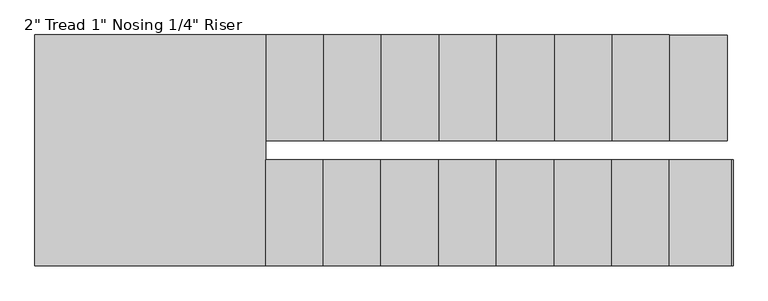
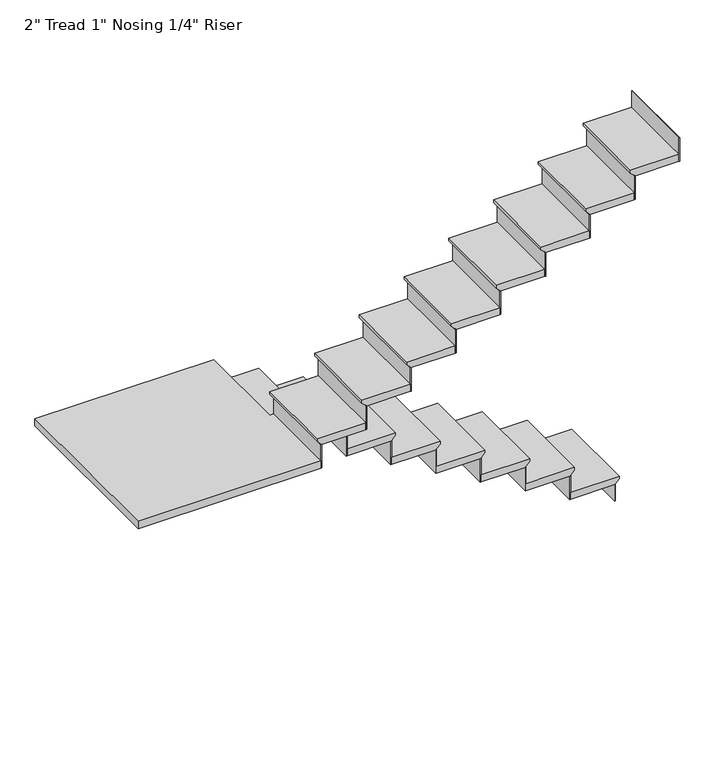
"""IFC4 building model written with IfcOpenShell, lengths in millimetres: stair flight geometry."""

from ifc_helpers import new_model, si_unit, origin, place, context, project, spatial, faceted_brep, source, transform, mapped, element, save


def stair_flight_719863f8(model_context):
    return source(origin(), model_context, "Body", "Brep", [
        faceted_brep([(-1805.9198569, -5306.3933037, 6551.0833333), (-1805.9198569, -5306.3933037, 6570.1333333), (-1805.9198569, -5865.1933037, 6570.1333333), (-1805.9198569, -5865.1933037, 6551.0833333), (-1831.3198569, -5306.3933037, 6525.6833333), (-1831.3198569, -5865.1933037, 6525.6833333), (-2136.1198569, -5306.3933037, 6570.1333333), (-2136.1198569, -5865.1933037, 6570.1333333), (-1831.3198569, -5865.1933037, 6519.3333333), (-2136.1198569, -5865.1933037, 6519.3333333), (-2136.1198569, -5306.3933037, 6519.3333333), (-1831.3198569, -5306.3933037, 6519.3333333)], [[[0, 1, 2, 3]], [[4, 0, 3, 5]], [[2, 1, 6, 7]], [[8, 9, 10, 11]], [[2, 7, 9, 8, 5, 3]], [[8, 11, 4, 5]], [[6, 1, 0, 4, 11, 10]], [[7, 6, 10, 9]]]),
        faceted_brep([(-1831.3198569, -5306.3933037, 6519.3333333), (-1831.3198569, -5306.3933037, 6400.8), (-1837.6698569, -5306.3933037, 6400.8), (-1837.6698569, -5306.3933037, 6519.3333333), (-1831.3198569, -5865.1933037, 6519.3333333), (-1837.6698569, -5865.1933037, 6519.3333333), (-1837.6698569, -5865.1933037, 6400.8), (-1831.3198569, -5865.1933037, 6400.8)], [[[0, 1, 2, 3]], [[4, 5, 6, 7]], [[1, 0, 4, 7]], [[2, 1, 7, 6]], [[3, 2, 6, 5]], [[0, 3, 5, 4]]]),
        faceted_brep([(-2136.1198569, -5306.3933037, 6688.6666667), (-2136.1198569, -5306.3933037, 6519.3333333), (-2142.4698569, -5306.3933037, 6519.3333333), (-2142.4698569, -5306.3933037, 6688.6666667), (-2136.1198569, -5865.1933037, 6688.6666667), (-2142.4698569, -5865.1933037, 6688.6666667), (-2142.4698569, -5865.1933037, 6519.3333333), (-2136.1198569, -5865.1933037, 6519.3333333)], [[[0, 1, 2, 3]], [[4, 5, 6, 7]], [[1, 0, 4, 7]], [[2, 1, 7, 6]], [[3, 2, 6, 5]], [[0, 3, 5, 4]]]),
        faceted_brep([(-2110.7198569, -5865.1933037, 6739.4666667), (-2110.7198569, -5306.3933037, 6739.4666667), (-2440.9198569, -5306.3933037, 6739.4666667), (-2440.9198569, -5865.1933037, 6739.4666667), (-2136.1198569, -5865.1933037, 6688.6666667), (-2440.9198569, -5865.1933037, 6688.6666667), (-2440.9198569, -5306.3933037, 6688.6666667), (-2136.1198569, -5306.3933037, 6688.6666667), (-2136.1198569, -5865.1933037, 6695.0166667), (-2110.7198569, -5865.1933037, 6720.4166667), (-2136.1198569, -5306.3933037, 6695.0166667), (-2110.7198569, -5306.3933037, 6720.4166667)], [[[0, 1, 2, 3]], [[4, 5, 6, 7]], [[0, 3, 5, 4, 8, 9]], [[4, 7, 10, 8]], [[2, 1, 11, 10, 7, 6]], [[3, 2, 6, 5]], [[11, 1, 0, 9]], [[10, 11, 9, 8]]]),
        faceted_brep([(-2440.9198569, -5306.3933037, 6858.0), (-2440.9198569, -5306.3933037, 6688.6666667), (-2447.2698569, -5306.3933037, 6688.6666667), (-2447.2698569, -5306.3933037, 6858.0), (-2440.9198569, -5865.1933037, 6858.0), (-2447.2698569, -5865.1933037, 6858.0), (-2447.2698569, -5865.1933037, 6688.6666667), (-2440.9198569, -5865.1933037, 6688.6666667)], [[[0, 1, 2, 3]], [[4, 5, 6, 7]], [[1, 0, 4, 7]], [[2, 1, 7, 6]], [[3, 2, 6, 5]], [[0, 3, 5, 4]]]),
        faceted_brep([(-2415.5198569, -5865.1933037, 6908.8), (-2415.5198569, -5306.3933037, 6908.8), (-2745.7198569, -5306.3933037, 6908.8), (-2745.7198569, -5865.1933037, 6908.8), (-2440.9198569, -5865.1933037, 6858.0), (-2745.7198569, -5865.1933037, 6858.0), (-2745.7198569, -5306.3933037, 6858.0), (-2440.9198569, -5306.3933037, 6858.0), (-2440.9198569, -5865.1933037, 6864.35), (-2415.5198569, -5865.1933037, 6889.75), (-2440.9198569, -5306.3933037, 6864.35), (-2415.5198569, -5306.3933037, 6889.75)], [[[0, 1, 2, 3]], [[4, 5, 6, 7]], [[0, 3, 5, 4, 8, 9]], [[4, 7, 10, 8]], [[2, 1, 11, 10, 7, 6]], [[3, 2, 6, 5]], [[11, 1, 0, 9]], [[10, 11, 9, 8]]]),
        faceted_brep([(-2745.7198569, -5306.3933037, 7027.3333333), (-2745.7198569, -5306.3933037, 6858.0), (-2752.0698569, -5306.3933037, 6858.0), (-2752.0698569, -5306.3933037, 7027.3333333), (-2745.7198569, -5865.1933037, 7027.3333333), (-2752.0698569, -5865.1933037, 7027.3333333), (-2752.0698569, -5865.1933037, 6858.0), (-2745.7198569, -5865.1933037, 6858.0)], [[[0, 1, 2, 3]], [[4, 5, 6, 7]], [[1, 0, 4, 7]], [[2, 1, 7, 6]], [[3, 2, 6, 5]], [[0, 3, 5, 4]]]),
        faceted_brep([(-2720.3198569, -5865.1933037, 7078.1333333), (-2720.3198569, -5306.3933037, 7078.1333333), (-3050.5198569, -5306.3933037, 7078.1333333), (-3050.5198569, -5865.1933037, 7078.1333333), (-2745.7198569, -5865.1933037, 7027.3333333), (-3050.5198569, -5865.1933037, 7027.3333333), (-3050.5198569, -5306.3933037, 7027.3333333), (-2745.7198569, -5306.3933037, 7027.3333333), (-2745.7198569, -5865.1933037, 7033.6833333), (-2720.3198569, -5865.1933037, 7059.0833333), (-2745.7198569, -5306.3933037, 7033.6833333), (-2720.3198569, -5306.3933037, 7059.0833333)], [[[0, 1, 2, 3]], [[4, 5, 6, 7]], [[0, 3, 5, 4, 8, 9]], [[4, 7, 10, 8]], [[2, 1, 11, 10, 7, 6]], [[3, 2, 6, 5]], [[11, 1, 0, 9]], [[10, 11, 9, 8]]]),
        faceted_brep([(-3050.5198569, -5306.3933037, 7196.6666667), (-3050.5198569, -5306.3933037, 7027.3333333), (-3056.8698569, -5306.3933037, 7027.3333333), (-3056.8698569, -5306.3933037, 7196.6666667), (-3050.5198569, -5865.1933037, 7196.6666667), (-3056.8698569, -5865.1933037, 7196.6666667), (-3056.8698569, -5865.1933037, 7027.3333333), (-3050.5198569, -5865.1933037, 7027.3333333)], [[[0, 1, 2, 3]], [[4, 5, 6, 7]], [[1, 0, 4, 7]], [[2, 1, 7, 6]], [[3, 2, 6, 5]], [[0, 3, 5, 4]]]),
        faceted_brep([(-3025.1198569, -5865.1933037, 7247.4666667), (-3025.1198569, -5306.3933037, 7247.4666667), (-3355.3198569, -5306.3933037, 7247.4666667), (-3355.3198569, -5865.1933037, 7247.4666667), (-3050.5198569, -5865.1933037, 7196.6666667), (-3355.3198569, -5865.1933037, 7196.6666667), (-3355.3198569, -5306.3933037, 7196.6666667), (-3050.5198569, -5306.3933037, 7196.6666667), (-3050.5198569, -5865.1933037, 7203.0166667), (-3025.1198569, -5865.1933037, 7228.4166667), (-3050.5198569, -5306.3933037, 7203.0166667), (-3025.1198569, -5306.3933037, 7228.4166667)], [[[0, 1, 2, 3]], [[4, 5, 6, 7]], [[0, 3, 5, 4, 8, 9]], [[4, 7, 10, 8]], [[2, 1, 11, 10, 7, 6]], [[3, 2, 6, 5]], [[11, 1, 0, 9]], [[10, 11, 9, 8]]]),
        faceted_brep([(-3355.3198569, -5306.3933037, 7366.0), (-3355.3198569, -5306.3933037, 7196.6666667), (-3361.6698569, -5306.3933037, 7196.6666667), (-3361.6698569, -5306.3933037, 7366.0), (-3355.3198569, -5865.1933037, 7366.0), (-3361.6698569, -5865.1933037, 7366.0), (-3361.6698569, -5865.1933037, 7196.6666667), (-3355.3198569, -5865.1933037, 7196.6666667)], [[[0, 1, 2, 3]], [[4, 5, 6, 7]], [[1, 0, 4, 7]], [[2, 1, 7, 6]], [[3, 2, 6, 5]], [[0, 3, 5, 4]]]),
        faceted_brep([(-3329.9198569, -5865.1933037, 7416.8), (-3329.9198569, -5306.3933037, 7416.8), (-3660.1198569, -5306.3933037, 7416.8), (-3660.1198569, -5865.1933037, 7416.8), (-3355.3198569, -5865.1933037, 7366.0), (-3660.1198569, -5865.1933037, 7366.0), (-3660.1198569, -5306.3933037, 7366.0), (-3355.3198569, -5306.3933037, 7366.0), (-3355.3198569, -5865.1933037, 7372.35), (-3329.9198569, -5865.1933037, 7397.75), (-3355.3198569, -5306.3933037, 7372.35), (-3329.9198569, -5306.3933037, 7397.75)], [[[0, 1, 2, 3]], [[4, 5, 6, 7]], [[0, 3, 5, 4, 8, 9]], [[4, 7, 10, 8]], [[2, 1, 11, 10, 7, 6]], [[3, 2, 6, 5]], [[11, 1, 0, 9]], [[10, 11, 9, 8]]]),
        faceted_brep([(-3660.1198569, -5306.3933037, 7535.3333333), (-3660.1198569, -5306.3933037, 7366.0), (-3666.4698569, -5306.3933037, 7366.0), (-3666.4698569, -5306.3933037, 7535.3333333), (-3660.1198569, -5865.1933037, 7535.3333333), (-3666.4698569, -5865.1933037, 7535.3333333), (-3666.4698569, -5865.1933037, 7366.0), (-3660.1198569, -5865.1933037, 7366.0)], [[[0, 1, 2, 3]], [[4, 5, 6, 7]], [[1, 0, 4, 7]], [[2, 1, 7, 6]], [[3, 2, 6, 5]], [[0, 3, 5, 4]]]),
        faceted_brep([(-3634.7198569, -5865.1933037, 7586.1333333), (-3634.7198569, -5306.3933037, 7586.1333333), (-3964.9198569, -5306.3933037, 7586.1333333), (-3964.9198569, -5865.1933037, 7586.1333333), (-3660.1198569, -5865.1933037, 7535.3333333), (-3964.9198569, -5865.1933037, 7535.3333333), (-3964.9198569, -5306.3933037, 7535.3333333), (-3660.1198569, -5306.3933037, 7535.3333333), (-3660.1198569, -5865.1933037, 7541.6833333), (-3634.7198569, -5865.1933037, 7567.0833333), (-3660.1198569, -5306.3933037, 7541.6833333), (-3634.7198569, -5306.3933037, 7567.0833333)], [[[0, 1, 2, 3]], [[4, 5, 6, 7]], [[0, 3, 5, 4, 8, 9]], [[4, 7, 10, 8]], [[2, 1, 11, 10, 7, 6]], [[3, 2, 6, 5]], [[11, 1, 0, 9]], [[10, 11, 9, 8]]]),
        faceted_brep([(-3964.9198569, -5306.3933037, 7704.6666667), (-3964.9198569, -5306.3933037, 7535.3333333), (-3971.2698569, -5306.3933037, 7535.3333333), (-3971.2698569, -5306.3933037, 7704.6666667), (-3964.9198569, -5865.1933037, 7704.6666667), (-3971.2698569, -5865.1933037, 7704.6666667), (-3971.2698569, -5865.1933037, 7535.3333333), (-3964.9198569, -5865.1933037, 7535.3333333)], [[[0, 1, 2, 3]], [[4, 5, 6, 7]], [[1, 0, 4, 7]], [[2, 1, 7, 6]], [[3, 2, 6, 5]], [[0, 3, 5, 4]]]),
        faceted_brep([(-3939.5198569, -5865.1933037, 7755.4666667), (-3939.5198569, -5306.3933037, 7755.4666667), (-4269.7198569, -5306.3933037, 7755.4666667), (-4269.7198569, -5865.1933037, 7755.4666667), (-3964.9198569, -5865.1933037, 7704.6666667), (-4269.7198569, -5865.1933037, 7704.6666667), (-4269.7198569, -5306.3933037, 7704.6666667), (-3964.9198569, -5306.3933037, 7704.6666667), (-3964.9198569, -5865.1933037, 7711.0166667), (-3939.5198569, -5865.1933037, 7736.4166667), (-3964.9198569, -5306.3933037, 7711.0166667), (-3939.5198569, -5306.3933037, 7736.4166667)], [[[0, 1, 2, 3]], [[4, 5, 6, 7]], [[0, 3, 5, 4, 8, 9]], [[4, 7, 10, 8]], [[2, 1, 11, 10, 7, 6]], [[3, 2, 6, 5]], [[11, 1, 0, 9]], [[10, 11, 9, 8]]]),
        faceted_brep([(-4269.7198569, -5306.3933037, 7874.0), (-4269.7198569, -5306.3933037, 7704.6666667), (-4276.0698569, -5306.3933037, 7704.6666667), (-4276.0698569, -5306.3933037, 7874.0), (-4269.7198569, -5865.1933037, 7874.0), (-4276.0698569, -5865.1933037, 7874.0), (-4276.0698569, -5865.1933037, 7704.6666667), (-4269.7198569, -5865.1933037, 7704.6666667)], [[[0, 1, 2, 3]], [[4, 5, 6, 7]], [[1, 0, 4, 7]], [[2, 1, 7, 6]], [[3, 2, 6, 5]], [[0, 3, 5, 4]]]),
        faceted_brep([(-4218.9198569, -5966.7933037, 7924.8), (-4244.3198569, -5966.7933037, 7924.8), (-4244.3198569, -5306.3933037, 7924.8), (-5463.5198569, -5306.3933037, 7924.8), (-5463.5198569, -6525.5933037, 7924.8), (-4218.9198569, -6525.5933037, 7924.8), (-4244.3198569, -5966.7933037, 7874.0), (-4218.9198569, -5966.7933037, 7874.0), (-4218.9198569, -6525.5933037, 7874.0), (-5463.5198569, -6525.5933037, 7874.0), (-5463.5198569, -5306.3933037, 7874.0), (-4269.7198569, -5306.3933037, 7874.0), (-4269.7198569, -5865.1933037, 7874.0), (-4244.3198569, -5865.1933037, 7874.0), (-4244.3198569, -5865.1933037, 7905.75), (-4244.3198569, -5306.3933037, 7905.75), (-4269.7198569, -5865.1933037, 7880.35), (-4269.7198569, -5306.3933037, 7880.35)], [[[0, 1, 2, 3, 4, 5]], [[6, 7, 8, 9, 10, 11, 12, 13]], [[1, 0, 7, 6]], [[2, 1, 6, 13, 14, 15]], [[13, 12, 16, 14]], [[12, 11, 17, 16]], [[3, 2, 15, 17, 11, 10]], [[4, 3, 10, 9]], [[5, 4, 9, 8]], [[0, 5, 8, 7]], [[17, 15, 14, 16]]]),
        faceted_brep([(-4218.9198569, -6525.5933037, 8043.3333333), (-4218.9198569, -6525.5933037, 7874.0), (-4212.5698569, -6525.5933037, 7874.0), (-4212.5698569, -6525.5933037, 8043.3333333), (-4218.9198569, -5966.7933037, 8043.3333333), (-4212.5698569, -5966.7933037, 8043.3333333), (-4212.5698569, -5966.7933037, 7874.0), (-4218.9198569, -5966.7933037, 7874.0)], [[[0, 1, 2, 3]], [[4, 5, 6, 7]], [[1, 0, 4, 7]], [[2, 1, 7, 6]], [[3, 2, 6, 5]], [[0, 3, 5, 4]]]),
        faceted_brep([(-4244.3198569, -5966.7933037, 8094.1333333), (-4244.3198569, -6525.5933037, 8094.1333333), (-3914.1198569, -6525.5933037, 8094.1333333), (-3914.1198569, -5966.7933037, 8094.1333333), (-4218.9198569, -5966.7933037, 8043.3333333), (-3914.1198569, -5966.7933037, 8043.3333333), (-3914.1198569, -6525.5933037, 8043.3333333), (-4218.9198569, -6525.5933037, 8043.3333333), (-4218.9198569, -5966.7933037, 8049.6833333), (-4244.3198569, -5966.7933037, 8075.0833333), (-4218.9198569, -6525.5933037, 8049.6833333), (-4244.3198569, -6525.5933037, 8075.0833333)], [[[0, 1, 2, 3]], [[4, 5, 6, 7]], [[0, 3, 5, 4, 8, 9]], [[4, 7, 10, 8]], [[2, 1, 11, 10, 7, 6]], [[3, 2, 6, 5]], [[11, 1, 0, 9]], [[10, 11, 9, 8]]]),
        faceted_brep([(-3914.1198569, -6525.5933037, 8212.6666667), (-3914.1198569, -6525.5933037, 8043.3333333), (-3907.7698569, -6525.5933037, 8043.3333333), (-3907.7698569, -6525.5933037, 8212.6666667), (-3914.1198569, -5966.7933037, 8212.6666667), (-3907.7698569, -5966.7933037, 8212.6666667), (-3907.7698569, -5966.7933037, 8043.3333333), (-3914.1198569, -5966.7933037, 8043.3333333)], [[[0, 1, 2, 3]], [[4, 5, 6, 7]], [[1, 0, 4, 7]], [[2, 1, 7, 6]], [[3, 2, 6, 5]], [[0, 3, 5, 4]]]),
        faceted_brep([(-3939.5198569, -5966.7933037, 8263.4666667), (-3939.5198569, -6525.5933037, 8263.4666667), (-3609.3198569, -6525.5933037, 8263.4666667), (-3609.3198569, -5966.7933037, 8263.4666667), (-3914.1198569, -5966.7933037, 8212.6666667), (-3609.3198569, -5966.7933037, 8212.6666667), (-3609.3198569, -6525.5933037, 8212.6666667), (-3914.1198569, -6525.5933037, 8212.6666667), (-3914.1198569, -5966.7933037, 8219.0166667), (-3939.5198569, -5966.7933037, 8244.4166667), (-3914.1198569, -6525.5933037, 8219.0166667), (-3939.5198569, -6525.5933037, 8244.4166667)], [[[0, 1, 2, 3]], [[4, 5, 6, 7]], [[0, 3, 5, 4, 8, 9]], [[4, 7, 10, 8]], [[2, 1, 11, 10, 7, 6]], [[3, 2, 6, 5]], [[11, 1, 0, 9]], [[10, 11, 9, 8]]]),
        faceted_brep([(-3609.3198569, -6525.5933037, 8382.0), (-3609.3198569, -6525.5933037, 8212.6666667), (-3602.9698569, -6525.5933037, 8212.6666667), (-3602.9698569, -6525.5933037, 8382.0), (-3609.3198569, -5966.7933037, 8382.0), (-3602.9698569, -5966.7933037, 8382.0), (-3602.9698569, -5966.7933037, 8212.6666667), (-3609.3198569, -5966.7933037, 8212.6666667)], [[[0, 1, 2, 3]], [[4, 5, 6, 7]], [[1, 0, 4, 7]], [[2, 1, 7, 6]], [[3, 2, 6, 5]], [[0, 3, 5, 4]]]),
        faceted_brep([(-3634.7198569, -5966.7933037, 8432.8), (-3634.7198569, -6525.5933037, 8432.8), (-3304.5198569, -6525.5933037, 8432.8), (-3304.5198569, -5966.7933037, 8432.8), (-3609.3198569, -5966.7933037, 8382.0), (-3304.5198569, -5966.7933037, 8382.0), (-3304.5198569, -6525.5933037, 8382.0), (-3609.3198569, -6525.5933037, 8382.0), (-3609.3198569, -5966.7933037, 8388.35), (-3634.7198569, -5966.7933037, 8413.75), (-3609.3198569, -6525.5933037, 8388.35), (-3634.7198569, -6525.5933037, 8413.75)], [[[0, 1, 2, 3]], [[4, 5, 6, 7]], [[0, 3, 5, 4, 8, 9]], [[4, 7, 10, 8]], [[2, 1, 11, 10, 7, 6]], [[3, 2, 6, 5]], [[11, 1, 0, 9]], [[10, 11, 9, 8]]]),
        faceted_brep([(-3304.5198569, -6525.5933037, 8551.3333333), (-3304.5198569, -6525.5933037, 8382.0), (-3298.1698569, -6525.5933037, 8382.0), (-3298.1698569, -6525.5933037, 8551.3333333), (-3304.5198569, -5966.7933037, 8551.3333333), (-3298.1698569, -5966.7933037, 8551.3333333), (-3298.1698569, -5966.7933037, 8382.0), (-3304.5198569, -5966.7933037, 8382.0)], [[[0, 1, 2, 3]], [[4, 5, 6, 7]], [[1, 0, 4, 7]], [[2, 1, 7, 6]], [[3, 2, 6, 5]], [[0, 3, 5, 4]]]),
        faceted_brep([(-3329.9198569, -5966.7933037, 8602.1333333), (-3329.9198569, -6525.5933037, 8602.1333333), (-2999.7198569, -6525.5933037, 8602.1333333), (-2999.7198569, -5966.7933037, 8602.1333333), (-3304.5198569, -5966.7933037, 8551.3333333), (-2999.7198569, -5966.7933037, 8551.3333333), (-2999.7198569, -6525.5933037, 8551.3333333), (-3304.5198569, -6525.5933037, 8551.3333333), (-3304.5198569, -5966.7933037, 8557.6833333), (-3329.9198569, -5966.7933037, 8583.0833333), (-3304.5198569, -6525.5933037, 8557.6833333), (-3329.9198569, -6525.5933037, 8583.0833333)], [[[0, 1, 2, 3]], [[4, 5, 6, 7]], [[0, 3, 5, 4, 8, 9]], [[4, 7, 10, 8]], [[2, 1, 11, 10, 7, 6]], [[3, 2, 6, 5]], [[11, 1, 0, 9]], [[10, 11, 9, 8]]]),
        faceted_brep([(-2999.7198569, -6525.5933037, 8720.6666667), (-2999.7198569, -6525.5933037, 8551.3333333), (-2993.3698569, -6525.5933037, 8551.3333333), (-2993.3698569, -6525.5933037, 8720.6666667), (-2999.7198569, -5966.7933037, 8720.6666667), (-2993.3698569, -5966.7933037, 8720.6666667), (-2993.3698569, -5966.7933037, 8551.3333333), (-2999.7198569, -5966.7933037, 8551.3333333)], [[[0, 1, 2, 3]], [[4, 5, 6, 7]], [[1, 0, 4, 7]], [[2, 1, 7, 6]], [[3, 2, 6, 5]], [[0, 3, 5, 4]]]),
        faceted_brep([(-3025.1198569, -5966.7933037, 8771.4666667), (-3025.1198569, -6525.5933037, 8771.4666667), (-2694.9198569, -6525.5933037, 8771.4666667), (-2694.9198569, -5966.7933037, 8771.4666667), (-2999.7198569, -5966.7933037, 8720.6666667), (-2694.9198569, -5966.7933037, 8720.6666667), (-2694.9198569, -6525.5933037, 8720.6666667), (-2999.7198569, -6525.5933037, 8720.6666667), (-2999.7198569, -5966.7933037, 8727.0166667), (-3025.1198569, -5966.7933037, 8752.4166667), (-2999.7198569, -6525.5933037, 8727.0166667), (-3025.1198569, -6525.5933037, 8752.4166667)], [[[0, 1, 2, 3]], [[4, 5, 6, 7]], [[0, 3, 5, 4, 8, 9]], [[4, 7, 10, 8]], [[2, 1, 11, 10, 7, 6]], [[3, 2, 6, 5]], [[11, 1, 0, 9]], [[10, 11, 9, 8]]]),
        faceted_brep([(-2694.9198569, -6525.5933037, 8890.0), (-2694.9198569, -6525.5933037, 8720.6666667), (-2688.5698569, -6525.5933037, 8720.6666667), (-2688.5698569, -6525.5933037, 8890.0), (-2694.9198569, -5966.7933037, 8890.0), (-2688.5698569, -5966.7933037, 8890.0), (-2688.5698569, -5966.7933037, 8720.6666667), (-2694.9198569, -5966.7933037, 8720.6666667)], [[[0, 1, 2, 3]], [[4, 5, 6, 7]], [[1, 0, 4, 7]], [[2, 1, 7, 6]], [[3, 2, 6, 5]], [[0, 3, 5, 4]]]),
        faceted_brep([(-2720.3198569, -5966.7933037, 8940.8), (-2720.3198569, -6525.5933037, 8940.8), (-2390.1198569, -6525.5933037, 8940.8), (-2390.1198569, -5966.7933037, 8940.8), (-2694.9198569, -5966.7933037, 8890.0), (-2390.1198569, -5966.7933037, 8890.0), (-2390.1198569, -6525.5933037, 8890.0), (-2694.9198569, -6525.5933037, 8890.0), (-2694.9198569, -5966.7933037, 8896.35), (-2720.3198569, -5966.7933037, 8921.75), (-2694.9198569, -6525.5933037, 8896.35), (-2720.3198569, -6525.5933037, 8921.75)], [[[0, 1, 2, 3]], [[4, 5, 6, 7]], [[0, 3, 5, 4, 8, 9]], [[4, 7, 10, 8]], [[2, 1, 11, 10, 7, 6]], [[3, 2, 6, 5]], [[11, 1, 0, 9]], [[10, 11, 9, 8]]]),
        faceted_brep([(-2390.1198569, -6525.5933037, 9059.3333333), (-2390.1198569, -6525.5933037, 8890.0), (-2383.7698569, -6525.5933037, 8890.0), (-2383.7698569, -6525.5933037, 9059.3333333), (-2390.1198569, -5966.7933037, 9059.3333333), (-2383.7698569, -5966.7933037, 9059.3333333), (-2383.7698569, -5966.7933037, 8890.0), (-2390.1198569, -5966.7933037, 8890.0)], [[[0, 1, 2, 3]], [[4, 5, 6, 7]], [[1, 0, 4, 7]], [[2, 1, 7, 6]], [[3, 2, 6, 5]], [[0, 3, 5, 4]]]),
        faceted_brep([(-2415.5198569, -5966.7933037, 9110.1333333), (-2415.5198569, -6525.5933037, 9110.1333333), (-2085.3198569, -6525.5933037, 9110.1333333), (-2085.3198569, -5966.7933037, 9110.1333333), (-2390.1198569, -5966.7933037, 9059.3333333), (-2085.3198569, -5966.7933037, 9059.3333333), (-2085.3198569, -6525.5933037, 9059.3333333), (-2390.1198569, -6525.5933037, 9059.3333333), (-2390.1198569, -5966.7933037, 9065.6833333), (-2415.5198569, -5966.7933037, 9091.0833333), (-2390.1198569, -6525.5933037, 9065.6833333), (-2415.5198569, -6525.5933037, 9091.0833333)], [[[0, 1, 2, 3]], [[4, 5, 6, 7]], [[0, 3, 5, 4, 8, 9]], [[4, 7, 10, 8]], [[2, 1, 11, 10, 7, 6]], [[3, 2, 6, 5]], [[11, 1, 0, 9]], [[10, 11, 9, 8]]]),
        faceted_brep([(-2085.3198569, -6525.5933037, 9228.6666667), (-2085.3198569, -6525.5933037, 9059.3333333), (-2078.9698569, -6525.5933037, 9059.3333333), (-2078.9698569, -6525.5933037, 9228.6666667), (-2085.3198569, -5966.7933037, 9228.6666667), (-2078.9698569, -5966.7933037, 9228.6666667), (-2078.9698569, -5966.7933037, 9059.3333333), (-2085.3198569, -5966.7933037, 9059.3333333)], [[[0, 1, 2, 3]], [[4, 5, 6, 7]], [[1, 0, 4, 7]], [[2, 1, 7, 6]], [[3, 2, 6, 5]], [[0, 3, 5, 4]]]),
        faceted_brep([(-1780.5198569, -6525.5933037, 9398.0), (-1780.5198569, -6525.5933037, 9228.6666667), (-1774.1698569, -6525.5933037, 9228.6666667), (-1774.1698569, -6525.5933037, 9398.0), (-1780.5198569, -5966.7933037, 9398.0), (-1774.1698569, -5966.7933037, 9398.0), (-1774.1698569, -5966.7933037, 9228.6666667), (-1780.5198569, -5966.7933037, 9228.6666667)], [[[0, 1, 2, 3]], [[4, 5, 6, 7]], [[1, 0, 4, 7]], [[2, 1, 7, 6]], [[3, 2, 6, 5]], [[0, 3, 5, 4]]]),
        faceted_brep([(-2110.7198569, -5966.7933037, 9279.4666667), (-2110.7198569, -6525.5933037, 9279.4666667), (-1780.5198569, -6525.5933037, 9279.4666667), (-1780.5198569, -5966.7933037, 9279.4666667), (-2085.3198569, -5966.7933037, 9228.6666667), (-1780.5198569, -5966.7933037, 9228.6666667), (-1780.5198569, -6525.5933037, 9228.6666667), (-2085.3198569, -6525.5933037, 9228.6666667), (-2085.3198569, -5966.7933037, 9235.0166667), (-2110.7198569, -5966.7933037, 9260.4166667), (-2085.3198569, -6525.5933037, 9235.0166667), (-2110.7198569, -6525.5933037, 9260.4166667)], [[[0, 1, 2, 3]], [[4, 5, 6, 7]], [[0, 3, 5, 4, 8, 9]], [[4, 7, 10, 8]], [[2, 1, 11, 10, 7, 6]], [[3, 2, 6, 5]], [[11, 1, 0, 9]], [[10, 11, 9, 8]]]),
    ])


if __name__ == "__main__":
    model = new_model("IFC4")
    model_context = context("Model", 3, world=origin())
    ifc_project = project(units=[si_unit("LENGTHUNIT", "METRE", prefix="MILLI")], contexts=[model_context])
    site = spatial("IfcSite", under=ifc_project)
    building = spatial("IfcBuilding", under=site)
    placement = place(None, origin())
    stair_flight_shape = stair_flight_719863f8(model_context)
    element("IfcStairFlight", 1, ObjectType="2\" Tread 1\" Nosing 1/4\" Riser", at=placement, inside=building, context=model_context, shape_type="MappedRepresentation", body=[
        mapped(stair_flight_shape, transform((0.0, 0.0, 0.0), x_axis=(1.0, 0.0, 0.0), y_axis=(0.0, 1.0, 0.0), z_axis=(0.0, 0.0, 1.0))),
    ])
    save(model, "model.ifc")
